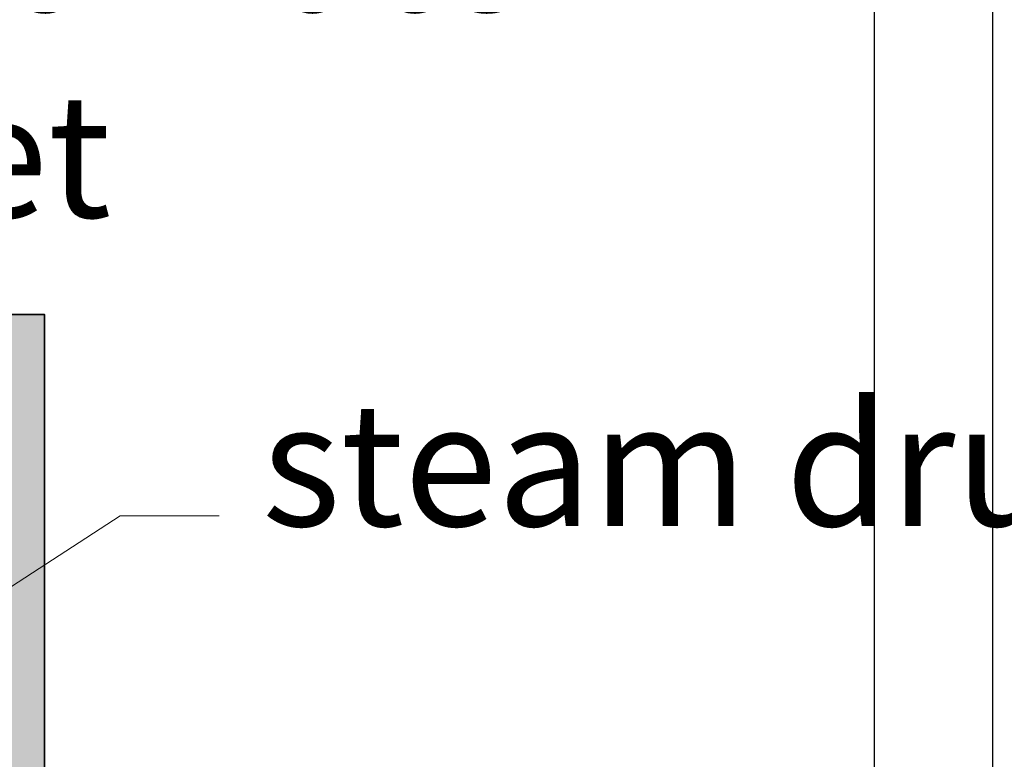
# Model space of a CAD drawing. Units: inches. Extents: x -1 to 292, y -3 to 199.
# Tile 42 of 52: x 181 to 220, y 101 to 131. Entities that reach past the tile are written whole.
import ezdxf

# ---------------------------------------------------------------- set-up
doc = ezdxf.new("R2010")
doc.units = ezdxf.units.IN
doc.header["$MEASUREMENT"] = 0
for name, color, linetype, lineweight in [('M-ANNO-LEAD', 2, 'Continuous', 18), ('M-ANNO-TEXT', 3, 'Continuous', 25), ('M-DIMS', 2, 'Continuous', 18), ('M-EQPM', 7, 'Continuous', 35), ('M-PATT', 8, 'Continuous', 13)]:
    doc.layers.add(name, color=color, linetype=linetype, lineweight=lineweight)
doc.styles.get("Standard").update_dxf_attribs({"font": 'arial.ttf'})
doc.dimstyles.get("Standard").update_dxf_attribs({"dimtxt": 0.18, "dimasz": 0.18, "dimexe": 0.18, "dimexo": 0.0625, "dimgap": 0.09, "dimtad": 0, "dimtih": 1, "dimtoh": 1, "dimdec": 4, "dimzin": 0, "dimdsep": 46, "dimtxsty": 'Standard', "dimcen": 0.09, "dimadec": 0, "dimazin": 0, "dimtfac": 1, "dimtdec": 4, "dimtofl": 0, "dimtmove": 0, "dimatfit": 3, "dimfxl": 1, "dimtolj": 1, "dimtzin": 0, "dimarcsym": 0})

# ---------------------------------------------------------------- blocks, each defined once
blk = doc.blocks.new('*D27')
at = {"layer": 'Defpoints', "color": 0, "transparency": 16777216}
for p in [(220.034, 174.363), (215.241, 88.13), (220.034, 85.363)]:
    blk.add_point(p, dxfattribs=at)
at = {"layer": 'M-DIMS', "color": 0, "lineweight": -2, "transparency": 16777216}
for p, q in [((215.241, 88.193), (215.241, 174.543)), ((220.034, 85.426), (220.034, 174.543)), ((215.421, 174.363), (217.24, 174.363)), ((219.854, 174.363), (218.035, 174.363))]:
    blk.add_line(p, q, dxfattribs=at)
at = {"layer": 'M-DIMS', "color": 0, "transparency": 16777216}
for points in [[(215.421, 174.393), (215.421, 174.333), (215.241, 174.363)], [(219.854, 174.393), (219.854, 174.333), (220.034, 174.363)]]:
    blk.add_solid(points, dxfattribs=at)
at = {"layer": 'M-DIMS', "color": 0, "transparency": 16777216, "insert": (217.637, 174.363), "char_height": 0.18, "attachment_point": 5}
blk.add_mtext('\\A1;4.793', dxfattribs=at)

msp = doc.modelspace()

# ---------------------------------------------------------------- hatches: boundary and pattern name
at = {"layer": 'M-PATT'}
h = msp.add_hatch(color=256, dxfattribs=at)
h.set_gradient(color1=(0, 127, 0), color2=(0, 127, 0), tint=1, name='CYLINDER')
h.paths.add_polyline_path([(164.5186, 119.2985), (129.9293, 119.2985), (129.9293, 117.2985), (164.1897, 117.2985)])
h.paths.add_polyline_path([(181.5897, 119.2985), (164.5186, 119.2985), (164.1897, 117.2985), (179.5897, 117.2985), (179.5897, 107.8518), (181.5897, 109.1506)])
h.paths.add_polyline_path([(181.5897, 109.1506), (179.5897, 107.8518), (179.5897, 36.2698), (198.4159, 36.2698), (198.4159, 38.2698), (181.5897, 38.2698)])
h.paths.add_polyline_path([(115.4883, 126.765), (111.4883, 126.765), (111.4883, 114.6589), (115.4883, 114.6589)])
h.paths.add_polyline_path([(123.408, 119.2985), (115.4883, 119.2985), (115.4883, 117.2985), (123.408, 117.2985)])
h.paths.add_polyline_path([(115.4883, 112.6589), (111.4883, 112.6589), (111.4883, 106.9941), (115.4883, 106.9941)])
h.paths.add_polyline_path([(120.9032, 106.9941), (106.0735, 106.9941), (106.0735, 105.9941), (120.9032, 105.9941)])
h.paths.add_polyline_path([(236.4209, 117.5104), (234.9209, 117.5104), (234.9209, 97.1861), (236.4209, 97.1861)])
h.paths.add_polyline_path([(236.4209, 126.4904), (234.9209, 126.4904), (234.9209, 118.9331), (236.4209, 118.9331)])
h.paths.add_polyline_path([(244.9552, 125.7269), (242.9552, 125.7269), (242.9552, 116.8562), (244.9552, 116.8562)])
h.paths.add_polyline_path([(244.9552, 115.1721), (242.9552, 115.1721), (242.9552, 109.7385), (244.9552, 109.7385)])
h.paths.add_polyline_path([(248.4468, 109.7385), (239.4637, 109.7385), (239.4637, 109.4289), (248.4468, 109.4289)])

# ---------------------------------------------------------------- linework, layer by layer
at = {"layer": 'M-ANNO-LEAD'}
for p, q in [((175.1158, 104.9464), (184.6596, 111.1442)), ((184.6596, 111.1442), (188.6815, 111.1442))]:
    msp.add_line(p, q, dxfattribs=at)
at = {"layer": 'M-EQPM'}
msp.add_lwpolyline([(129.9293, 119.2985), (181.5897, 119.2985), (181.5897, 38.2698)], dxfattribs=at)

# ---------------------------------------------------------------- texts
at = {"layer": 'M-ANNO-TEXT', "char_height": 5, "attachment_point": 1}
for s, insert in [('feed water inlet', (169.9729, 136.5612)), ('steam drum', (190.4016, 115.7236))]:
    msp.add_mtext_dynamic_manual_height_columns(s, width=47.899539, gutter_width=1, heights=[0], dxfattribs=dict(at, insert=insert))

# ---------------------------------------------------------------- dimensions: what is measured, and where the dimension line sits
at = {"layer": 'M-DIMS'}
dim = msp.add_linear_dim(base=(220.034, 174.3627), p1=(215.2407, 88.1304), p2=(220.034, 85.363), dimstyle='Standard', override={"dimdec": 3, "dimlfac": 1, "dimrnd": 0, "dimzin": 0, "dimdsep": 46, "dimlunit": 2}, dxfattribs=at)
dim.commit()
dim.dimension.update_dxf_attribs({"geometry": '*D27', "text_midpoint": (217.6374, 174.3627)})

doc.saveas('drawing.dxf')
